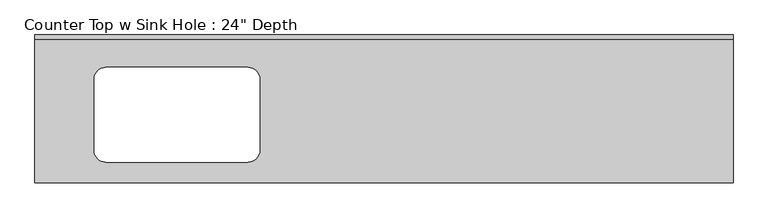
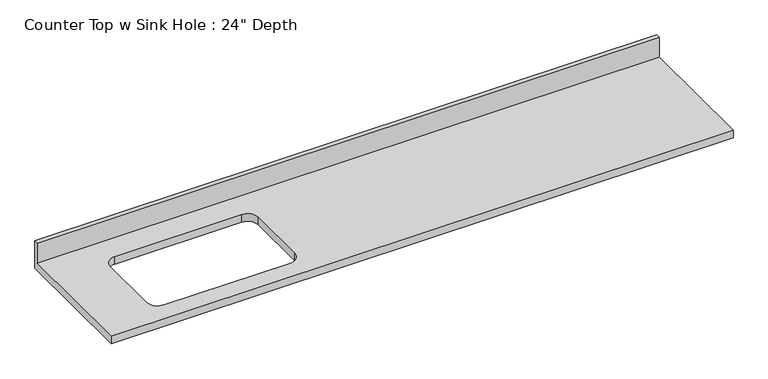
"""IFC4 building model written with IfcOpenShell, lengths in millimetres: furniture geometry."""

from ifc_helpers import new_model, si_unit, frame, origin, place, context, project, spatial, polyline, circle_curve, source, transform, mapped, element, save
from ifc_brep_helpers import plane_surface, revolved_surface, advanced_brep


def furniture_c0b61535(model_context):
    return source(origin(), model_context, "Body", "AdvancedBrep", [
        advanced_brep(
        [(-1200.4622951, -635.0, 914.4), (1796.7377049, -635.0, 914.4), (1796.7377049, -19.05, 914.4), (-1200.4622951, -19.05, 914.4), (-895.6622951, -139.7, 914.4), (-286.0622951, -139.7, 914.4), (-235.2622951, -190.5, 914.4), (-235.2622951, -495.3, 914.4), (-286.0622951, -546.1, 914.4), (-895.6622951, -546.1, 914.4), (-946.4622951, -495.3, 914.4), (-946.4622951, -190.5, 914.4), (1796.7377049, 0.0, 876.3), (1796.7377049, -635.0, 876.3), (-1200.4622951, -635.0, 876.3), (-1200.4622951, 0.0, 876.3), (-286.0622951, -139.7, 876.3), (-895.6622951, -139.7, 876.3), (-946.4622951, -190.5, 876.3), (-946.4622951, -495.3, 876.3), (-895.6622951, -546.1, 876.3), (-286.0622951, -546.1, 876.3), (-235.2622951, -495.3, 876.3), (-235.2622951, -190.5, 876.3), (-1200.4622951, 0.0, 1016.0), (1796.7377049, 0.0, 1016.0), (-1200.4622951, -19.05, 1016.0), (1796.7377049, -19.05, 1016.0)],
        [
            (0, 1),
            (1, 2),
            (2, 3),
            (3, 0),
            (4, 5),
            (5, 6, circle_curve(frame((-286.0622951, -190.5, 914.4), z_axis=(0.0, 0.0, -1.0), x_axis=(1.0, 0.0, 0.0)), 50.8)),
            (6, 7),
            (7, 8, circle_curve(frame((-286.0622951, -495.3, 914.4), z_axis=(0.0, 0.0, -1.0), x_axis=(1.0, 0.0, 0.0)), 50.8)),
            (8, 9),
            (9, 10, circle_curve(frame((-895.6622951, -495.3, 914.4), z_axis=(0.0, 0.0, -1.0), x_axis=(1.0, 0.0, 0.0)), 50.8)),
            (10, 11),
            (11, 4, circle_curve(frame((-895.6622951, -190.5, 914.4), z_axis=(0.0, 0.0, -1.0), x_axis=(1.0, 0.0, 0.0)), 50.8)),
            (12, 13),
            (13, 14),
            (14, 15),
            (15, 12),
            (16, 17),
            (17, 18, circle_curve(frame((-895.6622951, -190.5, 876.3), z_axis=(0.0, 0.0, 1.0), x_axis=(1.0, 0.0, 0.0)), 50.8)),
            (18, 19),
            (19, 20, circle_curve(frame((-895.6622951, -495.3, 876.3), z_axis=(0.0, 0.0, 1.0), x_axis=(1.0, 0.0, 0.0)), 50.8)),
            (20, 21),
            (21, 22, circle_curve(frame((-286.0622951, -495.3, 876.3), z_axis=(0.0, 0.0, 1.0), x_axis=(1.0, 0.0, 0.0)), 50.8)),
            (22, 23),
            (23, 16, circle_curve(frame((-286.0622951, -190.5, 876.3), z_axis=(0.0, 0.0, 1.0), x_axis=(1.0, 0.0, 0.0)), 50.8)),
            (15, 24),
            (24, 25),
            (25, 12),
            (14, 0),
            (3, 26),
            (26, 24),
            (13, 1),
            (25, 27),
            (27, 2),
            (26, 27),
            (4, 17),
            (16, 5),
            (11, 18),
            (10, 19),
            (9, 20),
            (8, 21),
            (7, 22),
            (6, 23),
        ],
        [
            plane_surface(frame((-1200.4622951, 0.0, 914.4), z_axis=(0.0, 0.0, 1.0), x_axis=(-1.0, 0.0, 0.0))),
            plane_surface(frame((-1200.4622951, 0.0, 876.3), z_axis=(0.0, 0.0, -1.0), x_axis=(1.0, 0.0, 0.0))),
            plane_surface(frame((1796.7377049, 0.0, 914.4), z_axis=(0.0, 1.0, 0.0), x_axis=(0.0, 0.0, -1.0))),
            plane_surface(frame((-1200.4622951, 0.0, 914.4), z_axis=(-1.0, 0.0, 0.0), x_axis=(0.0, 0.0, -1.0))),
            plane_surface(frame((-1200.4622951, -635.0, 914.4), z_axis=(0.0, -1.0, 0.0), x_axis=(0.0, 0.0, -1.0))),
            plane_surface(frame((1796.7377049, -635.0, 914.4), z_axis=(1.0, 0.0, 0.0), x_axis=(0.0, 0.0, -1.0))),
            plane_surface(frame((-1200.4622951, 0.0, 1016.0), z_axis=(0.0, 0.0, 1.0), x_axis=(0.0, -1.0, 0.0))),
            plane_surface(frame((-1200.4622951, -19.05, 1016.0), z_axis=(0.0, -1.0, 0.0), x_axis=(0.0, 0.0, -1.0))),
            plane_surface(frame((-286.0622951, -139.7, 914.4), z_axis=(0.0, -1.0, 0.0), x_axis=(0.0, 0.0, -1.0))),
            revolved_surface(polyline([(-844.8622951000001, -190.5, 914.4), (-844.8622951000001, -190.5, 876.3)]), (-895.6622951, -190.5, 876.3), (0.0, 0.0, 1.0)),
            plane_surface(frame((-946.4622951, -190.5, 914.4), z_axis=(1.0, 0.0, 0.0), x_axis=(0.0, 0.0, -1.0))),
            revolved_surface(polyline([(-844.8622951000001, -495.3, 914.4), (-844.8622951000001, -495.3, 876.3)]), (-895.6622951, -495.3, 876.3), (0.0, 0.0, 1.0)),
            plane_surface(frame((-895.6622951, -546.1, 914.4), z_axis=(0.0, 1.0, 0.0), x_axis=(0.0, 0.0, -1.0))),
            revolved_surface(polyline([(-235.26229509999996, -495.3, 914.4), (-235.26229509999996, -495.3, 876.3)]), (-286.0622951, -495.3, 876.3), (0.0, 0.0, 1.0)),
            plane_surface(frame((-235.2622951, -495.3, 914.4), z_axis=(-1.0, 0.0, 0.0), x_axis=(0.0, 0.0, -1.0))),
            revolved_surface(polyline([(-235.26229509999996, -190.5, 914.4), (-235.26229509999996, -190.5, 876.3)]), (-286.0622951, -190.5, 876.3), (0.0, 0.0, 1.0)),
        ],
        [
            (0, [[1, 2, 3, 4], [5, 6, 7, 8, 9, 10, 11, 12]]),
            (1, [[13, 14, 15, 16], [17, 18, 19, 20, 21, 22, 23, 24]]),
            (2, [[-16, 25, 26, 27]]),
            (3, [[-15, 28, -4, 29, 30, -25]]),
            (4, [[-1, -28, -14, 31]]),
            (5, [[-13, -27, 32, 33, -2, -31]]),
            (6, [[-30, 34, -32, -26]]),
            (7, [[-34, -29, -3, -33]]),
            (8, [[35, -17, 36, -5]]),
            (9, [[-35, -12, 37, -18]]),
            (10, [[-37, -11, 38, -19]]),
            (11, [[-38, -10, 39, -20]]),
            (12, [[-39, -9, 40, -21]]),
            (13, [[-40, -8, 41, -22]]),
            (14, [[-41, -7, 42, -23]]),
            (15, [[-36, -24, -42, -6]]),
        ],
    ),
    ])


if __name__ == "__main__":
    model = new_model("IFC4")
    model_context = context("Model", 3, world=origin())
    ifc_project = project(units=[si_unit("LENGTHUNIT", "METRE", prefix="MILLI")], contexts=[model_context])
    site = spatial("IfcSite", under=ifc_project)
    building = spatial("IfcBuilding", under=site)
    placement = place(None, origin())
    furniture_shape = furniture_c0b61535(model_context)
    element("IfcFurniture", 1, ObjectType="Counter Top w Sink Hole : 24\" Depth", at=placement, inside=building, context=model_context, shape_type="MappedRepresentation", body=[
        mapped(furniture_shape, transform((0.0, 0.0, 0.0), x_axis=(1.0, 0.0, 0.0), y_axis=(0.0, 1.0, 0.0), z_axis=(0.0, 0.0, 1.0))),
    ])
    save(model, "model.ifc")

# Revit data of these elements
# Type "Counter Top w Sink Hole : 24\" Depth"
#   Assembly Code = "C1030400"
#   Counter Thickness = 0' - 1 1/2"
#   Depth = 2' - 1"
#   Height = 3' - 0"
#   Length [instance default] = 8' - 0"
#   Sink Location [instance default] = 2' - 0"
#   Sink Location To Wall [instance default] = 0' - 6"
#   Sink Opening Depth [instance default] = 1' - 3"
#   Sink Opening Width [instance default] = 2' - 3"
#   Counter Top Material = none
#   Default Elevation = 0
# Element 1 (IfcFurniture, "Counter Top w Sink Hole : 24\" Depth")
#   Length = 9' - 10"
#   Materials on its faces: "Counter Top"
# Materials
#   "Counter Top": class "Wood", colour RGB 226 177 128, transparency 0
